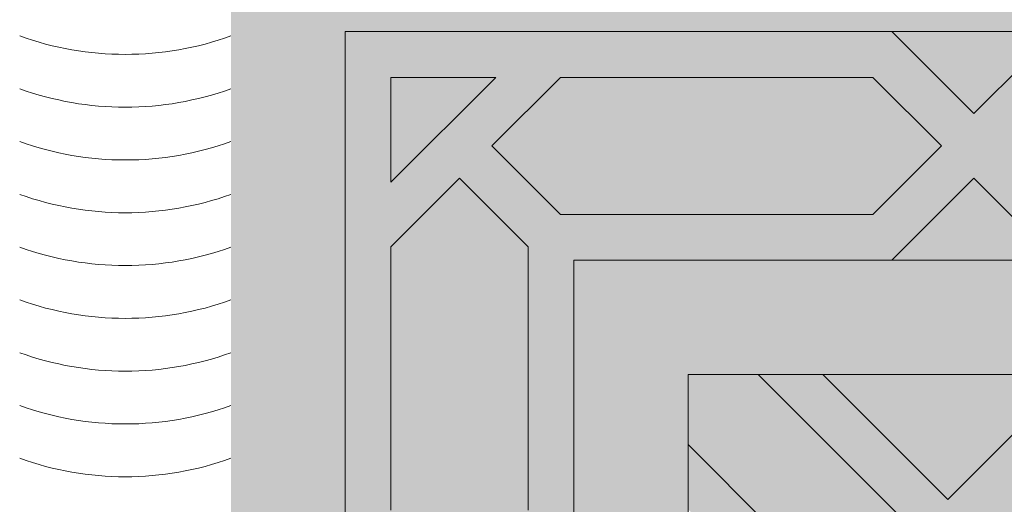
# Model space of a CAD drawing. Units: inches. Extents: x 844 to 2234, y 346 to 1084.
# Tile 58 of 93: x 1861.148 to 1866.641, y 710.205 to 712.909. Entities that reach past the tile are written whole.
import ezdxf

# ---------------------------------------------------------------- set-up
doc = ezdxf.new("R2010")
doc.units = ezdxf.units.IN
doc.header["$MEASUREMENT"] = 0
doc.layers.add('furniture', color=8, linetype='Continuous', lineweight=18)
doc.layers.add('RA-AP-01$0$INT', color=35, linetype='Continuous', lineweight=5)
doc.layers.add('RA-AP-01$0$FURN', color=3, linetype='Continuous')

# ---------------------------------------------------------------- blocks, each defined once
blk = doc.blocks.new('A$C18D01794')
at = {"layer": 'RA-AP-01$0$INT'}
h = blk.add_hatch(color=256, dxfattribs=at)
h.paths.add_polyline_path([(4.355206456958071, -6.156712009588037), (4.355206456958071, -8.056712009588038), (5.455206456958072, -8.056712009588038), (5.455206456958072, -6.156712009588037)])
h.paths.add_polyline_path([(4.405206456958072, -8.006712009588039), (4.405206456958072, -6.206712009588038), (5.405206456958072, -6.206712009588038), (5.405206456958072, -8.006712009588039)], flags=16)
h = blk.add_hatch(color=256, dxfattribs=at)
h.paths.add_polyline_path([(4.505206456958071, -7.585498806127123), (4.46934859260189, -7.549640941759413), (4.505206456958071, -7.513783077414768), (4.505206456958071, -7.381963272220687), (4.469348592616735, -7.346105407867824), (4.505206456958071, -7.310247543514964), (4.505206456958071, -7.178427738324996), (4.469348592586679, -7.142569873965138), (4.505206456952245, -7.106712009588038), (4.476922185709333, -7.106712009588038), (4.455206456960671, -7.128427738343681), (4.433490728198047, -7.106712009588038), (4.405206456946033, -7.106712009588036), (4.441064321339216, -7.142569873969684), (4.40520645695807, -7.178427738362358), (4.405206456958072, -7.310247543472698), (4.441064321364728, -7.346105407867826), (4.40520645695807, -7.381963272262947), (4.40520645695807, -7.513783077378263), (4.441064321354429, -7.549640941786153), (4.405206456958072, -7.585498806170974), (4.405206456958072, -7.717318611286652), (4.441064321333084, -7.753176475673194), (4.405206456958072, -7.789034340036673), (4.405206456958072, -8.006712009588039), (4.644348592588106, -8.006712009588039), (4.680206456964639, -7.970854145211967), (4.716064321341165, -8.006712009588039), (4.869348592586113, -8.006712009588039), (4.905206456964143, -7.970854145210465), (4.941064321342174, -8.006712009588039), (5.094348592587118, -8.006712009588037), (5.130206456963649, -7.970854145211967), (5.166064321340178, -8.006712009588039), (5.405206456958072, -8.006712009588039), (5.405206456958072, -7.789034340024526), (5.369348592595202, -7.753176475673196), (5.40520645695807, -7.717318611298797), (5.40520645695807, -7.585498806158829), (5.369348592573859, -7.549640941786151), (5.40520645695807, -7.51378307739041), (5.40520645695807, -7.381963272250803), (5.36934859256356, -7.346105407867824), (5.405206456958072, -7.310247543484846), (5.405206456958072, -7.178427738350217), (5.369348592589068, -7.142569873969682), (5.405206456982249, -7.106712009588038), (5.376922185730244, -7.106712009588038), (5.355206456967613, -7.128427738343679), (5.333490728218955, -7.10671200958804), (5.305206456976043, -7.106712009588042), (5.341064321341609, -7.142569873965136), (5.305206456958072, -7.178427738337141), (5.305206456958072, -7.310247543502816), (5.34106432131155, -7.346105407867824), (5.305206456958072, -7.381963272232832), (5.30520645695807, -7.513783077402624), (5.341064321326395, -7.549640941759413), (5.305206456958072, -7.585498806139263), (5.305206456958072, -7.717318611299605), (5.341064321347738, -7.753176475677737), (5.305206456958072, -7.78903434007894), (5.30520645695807, -7.906712009588039), (5.166064321336834, -7.906712009588039), (5.130206456963647, -7.942569873961684), (5.094348592590464, -7.906712009588039), (4.941064321338827, -7.906712009588041), (4.905206456964145, -7.942569873963183), (4.869348592589459, -7.906712009588039), (4.716064321337822, -7.906712009588041), (4.680206456964641, -7.942569873961684), (4.644348592591453, -7.906712009588039), (4.505206456958071, -7.906712009588039), (4.505206456958071, -7.789034340066795), (4.469348592580545, -7.753176475677738), (4.505206456958071, -7.717318611311748)])
h.paths.add_polyline_path([(4.485206456974132, -7.709034340046354), (4.45520645695909, -7.739034340051736), (4.425206456974128, -7.709034340057131), (4.425206456993394, -7.593783077384998), (4.45520645699153, -7.563783077396511), (4.485206456993396, -7.593783077408017)], flags=16)
h.paths.add_polyline_path([(4.455206456954537, -7.767318611299197), (4.485206456958242, -7.797318611312542), (4.48520645695951, -7.912569873958716), (4.45520645695415, -7.942569873954422), (4.425206456957888, -7.912569873967813), (4.425206456957888, -7.797318611286197)], flags=16)
h.paths.add_polyline_path([(4.455206456964794, -7.535498806149051), (4.42520645696469, -7.5054988061393), (4.425206456983954, -7.390247543486406), (4.455206456990734, -7.360247543489279), (4.485206456983953, -7.39024754349214), (4.485206456964687, -7.505498806158811)], flags=16)
h.paths.add_polyline_path([(4.499348592588947, -7.926712009585049), (4.636064321340932, -7.926712009585049), (4.666064321342317, -7.956712009586821), (4.636064321343707, -7.986712009585048), (4.499348592575121, -7.986712009585048), (4.469348592591685, -7.956712009591957)], flags=16)
h.paths.add_polyline_path([(4.425206456957888, -7.940854145195974), (4.471064321332215, -7.986712009585049), (4.425206456957888, -7.986712009585049)], flags=16)
h.paths.add_polyline_path([(4.455206456990734, -7.331963272246367), (4.425206456989053, -7.301963272254337), (4.425206456969784, -7.186712009596224), (4.455206456965226, -7.156712009591144), (4.485206456969787, -7.186712009586051), (4.485206456989053, -7.301963272238404)], flags=16)
h.paths.add_polyline_path([(4.72434859258714, -7.926712009586255), (4.861064321340141, -7.926712009586248), (4.891064321340324, -7.956712009586823), (4.861064321340513, -7.986712009586252), (4.724348592586768, -7.986712009586252), (4.694348592586956, -7.956712009586821)], flags=16)
h.paths.add_polyline_path([(4.919348592587961, -7.956712009586821), (4.949348592588145, -7.92671200958625), (5.08606432134115, -7.926712009586253), (5.116064321341327, -7.956712009586823), (5.086064321341519, -7.986712009586252), (4.949348592587774, -7.986712009586252)], flags=16)
h.paths.add_polyline_path([(5.144348592585967, -7.956712009586823), (5.174348592587358, -7.926712009585049), (5.311064321339338, -7.926712009585049), (5.3410643213366, -7.956712009591957), (5.311064321353163, -7.986712009585048), (5.174348592584576, -7.986712009585048)], flags=16)
h.paths.add_polyline_path([(5.32520645693489, -7.593783077408021), (5.355206456936755, -7.563783077396511), (5.385206456934894, -7.593783077384998), (5.38520645695416, -7.709034340057128), (5.355206456969194, -7.739034340051736), (5.325206456954153, -7.709034340046352)], flags=16)
h.paths.add_polyline_path([(5.325206456970042, -7.797318611312542), (5.355206456973747, -7.767318611299197), (5.385206456970398, -7.7973186112862), (5.385206456970398, -7.912569873967816), (5.355206456974136, -7.942569873954422), (5.325206456968778, -7.912569873958716)], flags=16)
h.paths.add_polyline_path([(5.325206456963599, -7.505498806158811), (5.325206456944333, -7.39024754349214), (5.355206456937552, -7.360247543489279), (5.385206456944332, -7.39024754348641), (5.385206456963596, -7.505498806139303), (5.355206456963492, -7.53549880614905)], flags=16)
h.paths.add_polyline_path([(5.32520645693923, -7.301963272238403), (5.3252064569585, -7.186712009586051), (5.355206456963062, -7.156712009591142), (5.3852064569585, -7.186712009596224), (5.385206456939234, -7.301963272254338), (5.355206456937552, -7.331963272246369)], flags=16)
h.paths.add_polyline_path([(5.339348592596071, -7.986712009585048), (5.385206456970398, -7.940854145195972), (5.385206456970396, -7.986712009585048)], flags=16)
h = blk.add_hatch(color=256, dxfattribs=at)
h.paths.add_polyline_path([(4.469348592586677, -7.142569873965136), (4.505206456958073, -7.178427738324996), (4.505206456958071, -7.106712009582215)])
h.paths.add_polyline_path([(4.455206456960671, -7.128427738343681), (4.476922185709333, -7.106712009588038), (4.433490728198045, -7.106712009588038)])
h.paths.add_polyline_path([(4.405206456958073, -7.178427738362358), (4.441064321339218, -7.142569873969684), (4.40520645695807, -7.106712009600073)])
h.paths.add_polyline_path([(4.425206456989053, -7.301963272254335), (4.455206456990736, -7.331963272246371), (4.485206456989055, -7.301963272238399), (4.48520645696979, -7.186712009586054), (4.455206456965227, -7.15671200959114), (4.425206456969784, -7.186712009596224)])
h.paths.add_polyline_path([(4.505206456958073, -7.381963272220689), (4.505206456958071, -7.310247543514961), (4.469348592616738, -7.346105407867826)])
h.paths.add_polyline_path([(4.425206456964688, -7.5054988061393), (4.455206456964794, -7.535498806149051), (4.485206456964689, -7.505498806158811), (4.485206456983951, -7.390247543492138), (4.455206456990736, -7.360247543489277), (4.425206456983956, -7.39024754348641)])
h.paths.add_polyline_path([(4.425206456974126, -7.709034340057128), (4.455206456959092, -7.739034340051736), (4.485206456974132, -7.709034340046356), (4.485206456993396, -7.593783077408017), (4.45520645699153, -7.563783077396511), (4.425206456993394, -7.593783077384999)])
h.paths.add_polyline_path([(4.46934859260189, -7.549640941759415), (4.505206456958071, -7.585498806127123), (4.505206456958073, -7.513783077414766)])
h.paths.add_polyline_path([(4.405206456958073, -7.585498806170972), (4.441064321354427, -7.549640941786151), (4.405206456958072, -7.513783077378263)])
h.paths.add_polyline_path([(4.405206456958072, -7.789034340036673), (4.441064321333084, -7.753176475673194), (4.405206456958072, -7.71731861128665)])
h.paths.add_polyline_path([(4.469348592580547, -7.75317647567774), (4.505206456958071, -7.789034340066795), (4.505206456958071, -7.717318611311744)])
h.paths.add_polyline_path([(4.425206456957888, -7.912569873967814), (4.45520645695415, -7.942569873954422), (4.485206456959507, -7.912569873958718), (4.48520645695824, -7.797318611312542), (4.455206456954537, -7.767318611299197), (4.425206456957888, -7.797318611286202)])
h.paths.add_polyline_path([(4.425206456957888, -7.986712009585049), (4.471064321332215, -7.986712009585049), (4.425206456957888, -7.940854145195972)])
h.paths.add_polyline_path([(4.499348592575121, -7.986712009585048), (4.636064321343707, -7.986712009585049), (4.666064321342317, -7.956712009586823), (4.636064321340932, -7.926712009585049), (4.499348592588945, -7.926712009585049), (4.469348592591685, -7.95671200959196)])
h.paths.add_polyline_path([(4.680206456964641, -7.942569873961684), (4.716064321337824, -7.906712009588039), (4.644348592591454, -7.906712009588039)])
h.paths.add_polyline_path([(4.644348592588108, -8.006712009588039), (4.716064321341167, -8.006712009588039), (4.680206456964637, -7.970854145211964)])
h.paths.add_polyline_path([(4.724348592586768, -7.98671200958625), (4.861064321340514, -7.986712009586252), (4.891064321340324, -7.956712009586819), (4.861064321340141, -7.92671200958625), (4.724348592587134, -7.926712009586255), (4.694348592586957, -7.956712009586821)])
h.paths.add_polyline_path([(4.905206456964143, -7.942569873963183), (4.941064321338827, -7.906712009588039), (4.869348592589457, -7.906712009588037)])
h.paths.add_polyline_path([(4.869348592586113, -8.006712009588039), (4.941064321342172, -8.006712009588037), (4.905206456964145, -7.970854145210463)])
h.paths.add_polyline_path([(4.949348592587774, -7.986712009586252), (5.086064321341521, -7.986712009586252), (5.116064321341329, -7.956712009586823), (5.08606432134115, -7.926712009586253), (4.949348592588145, -7.92671200958625), (4.919348592587961, -7.956712009586819)])
h.paths.add_polyline_path([(5.130206456963645, -7.942569873961684), (5.166064321336834, -7.906712009588039), (5.094348592590464, -7.906712009588039)])
h.paths.add_polyline_path([(5.094348592587119, -8.006712009588039), (5.166064321340178, -8.006712009588039), (5.130206456963651, -7.970854145211967)])
h.paths.add_polyline_path([(5.174348592584578, -7.986712009585048), (5.311064321353163, -7.986712009585048), (5.341064321336602, -7.956712009591958), (5.31106432133934, -7.926712009585049), (5.174348592587352, -7.926712009585049), (5.144348592585969, -7.956712009586823)])
h.paths.add_polyline_path([(5.325206456968778, -7.912569873958718), (5.355206456974136, -7.942569873954422), (5.385206456970396, -7.912569873967814), (5.385206456970396, -7.797318611286199), (5.355206456973747, -7.767318611299197), (5.325206456970044, -7.797318611312544)])
h.paths.add_polyline_path([(5.339348592596073, -7.986712009585048), (5.385206456970396, -7.986712009585049), (5.385206456970398, -7.94085414519597)])
h.paths.add_polyline_path([(5.325206456954155, -7.709034340046354), (5.355206456969194, -7.739034340051734), (5.38520645695416, -7.709034340057128), (5.385206456934896, -7.593783077384999), (5.355206456936758, -7.563783077396513), (5.325206456934888, -7.593783077408019)])
h.paths.add_polyline_path([(5.305206456958072, -7.789034340078938), (5.341064321347739, -7.753176475677738), (5.305206456958072, -7.717318611299605)])
h.paths.add_polyline_path([(5.369348592595204, -7.753176475673194), (5.40520645695807, -7.789034340024526), (5.405206456958072, -7.717318611298798)])
h.paths.add_polyline_path([(5.405206456958072, -7.585498806158831), (5.405206456958072, -7.513783077390407), (5.369348592573857, -7.549640941786151)])
h.paths.add_polyline_path([(5.305206456958072, -7.585498806139266), (5.341064321326393, -7.549640941759413), (5.305206456958072, -7.513783077402626)])
h.paths.add_polyline_path([(5.325206456963599, -7.50549880615881), (5.355206456963494, -7.535498806149055), (5.385206456963598, -7.505498806139302), (5.385206456944334, -7.390247543486411), (5.355206456937552, -7.360247543489279), (5.325206456944333, -7.39024754349214)])
h.paths.add_polyline_path([(5.305206456958072, -7.38196327223283), (5.341064321311551, -7.346105407867824), (5.305206456958072, -7.31024754350282)])
h.paths.add_polyline_path([(5.325206456939231, -7.301963272238404), (5.355206456937552, -7.331963272246369), (5.385206456939235, -7.301963272254335), (5.385206456958502, -7.186712009596224), (5.355206456963061, -7.156712009591142), (5.3252064569585, -7.186712009586051)])
h.paths.add_polyline_path([(5.404581768715993, -7.381338584008926, -0.001217816984214), (5.405206456958072, -7.381112009582329), (5.405206456958072, -7.310247543484846), (5.369348592563558, -7.346105407867826)])
h.paths.add_polyline_path([(5.36934859258907, -7.142569873969684), (5.40520645695807, -7.178427738350215), (5.405206456958072, -7.106712009612218)])
h.paths.add_polyline_path([(5.355206456967613, -7.128427738343683), (5.376922185730239, -7.106712009588038), (5.333490728218953, -7.10671200958804)])
h.paths.add_polyline_path([(5.30520645695807, -7.178427738337139), (5.341064321341609, -7.142569873965134), (5.305206456958074, -7.10671200957007)])
blk.add_hatch(color=256, dxfattribs=at).paths.add_polyline_path([(4.505206456958071, -7.906712009588039), (5.305206456958072, -7.906712009588039), (5.305206456958072, -7.106712009588038), (5.255206456951893, -7.106712009588036), (5.25520645694868, -7.856712009570104), (4.555206456959269, -7.856712009588616), (4.555206456956052, -7.106712009588038), (4.505206456958073, -7.106712009588038)])
h = blk.add_hatch(color=256, dxfattribs=at)
h.paths.add_polyline_path([(4.585917135068448, -7.856712009587804), (4.614201406330596, -7.856712009587056), (4.668846067270487, -7.802067348644738), (4.723490728212344, -7.856712009584164), (4.771774999457151, -7.856712009582887), (4.826419660396886, -7.80206734864072), (4.862780050090322, -7.838427738332541), (4.844495778842715, -7.856712009580965), (4.862780050090411, -7.856712009580482), (4.905206456960182, -7.814285602707865), (4.947632863832445, -7.856712009578238), (4.965917135079675, -7.856712009577755), (4.947632863831759, -7.838427738330656), (4.983993253523576, -7.802067348637219), (5.038637914464627, -7.856712009575829), (5.08692218571208, -7.856712009574554), (5.141566846649976, -7.802067348634224), (5.196211507589851, -7.856712009571666), (5.224495778822615, -7.856712009570916), (4.905206456953975, -7.537422687702283)])
h.paths.add_polyline_path([(4.895206456956031, -7.575706958950402), (4.895206456958921, -7.684996280828174), (4.840561796018589, -7.630351619890275)], flags=16)
h.paths.add_polyline_path([(4.915206456955638, -7.575706958949956), (4.969851117895509, -7.630351619887399), (4.915206456957609, -7.684996280827732)], flags=16)
h.paths.add_polyline_path([(4.826419660395175, -7.644493755514321), (4.881064321335613, -7.699138416452331), (4.771774999456703, -7.69913841645522)], flags=16)
h.paths.add_polyline_path([(4.983993253519558, -7.644493755510815), (5.038637914460456, -7.699138416449285), (4.929348592581548, -7.69913841645126)], flags=16)
h.paths.add_polyline_path([(4.881064321336025, -7.719138416452334), (4.826419660397532, -7.773783077393256), (4.771774999457062, -7.719138416455217)], flags=16)
h.paths.add_polyline_path([(4.929348592582019, -7.71913841645126), (5.038637914460982, -7.719138416449284), (4.983993253522945, -7.773783077389749)], flags=16)
h.paths.add_polyline_path([(4.895206456960191, -7.733280552075633), (4.895206456962115, -7.806001331460164), (4.876922185715016, -7.824285602708492), (4.840561796021581, -7.787925213016675)], flags=16)
h.paths.add_polyline_path([(4.915206456958487, -7.733280552075187), (4.969851117899527, -7.787925213013798), (4.933490728206909, -7.824285602708034), (4.9152064569598, -7.806001331461736)], flags=16)
h.paths.add_polyline_path([(4.757632863832376, -7.733280552079264), (4.812277524772842, -7.787925213017304), (4.757632863834348, -7.842569873958233)], flags=16)
h.paths.add_polyline_path([(4.737632863832376, -7.73328055207979), (4.737632863834348, -7.842569873958701), (4.682988202893906, -7.787925213020692)], flags=16)
h.paths.add_polyline_path([(5.05278005008503, -7.733280552072701), (5.052780050087917, -7.842569873951664), (4.998135389146995, -7.787925213013169)], flags=16)
h.paths.add_polyline_path([(5.072780050085024, -7.733280552072333), (5.127424711025931, -7.787925213010806), (5.072780050087916, -7.842569873951244)], flags=16)
h.paths.add_polyline_path([(4.935917135072783, -7.506712009583784), (5.255206456948811, -7.826001331459767), (5.255206456948932, -7.797717060211899), (5.200561796010279, -7.743072399273238), (5.255206456949403, -7.688427738334128), (5.25520645694961, -7.640143467086677), (5.200561796009787, -7.585498806146837), (5.236922185702417, -7.549138416454212), (5.255206456949919, -7.56742268770172), (5.255206456949998, -7.549138416454178), (5.212780050078687, -7.506712009583814), (5.25520645695036, -7.464285602712145), (5.255206456950438, -7.446001331464763), (5.236922185702424, -7.464285602712779), (5.200561796009796, -7.427925213020149), (5.255206456950753, -7.373280552079203), (5.25520645695096, -7.324996280834394), (5.200561796010322, -7.270351619893748), (5.255206456951428, -7.215706958952649), (5.255206456951547, -7.187422687705071)])
h.paths.add_polyline_path([(5.042988202883395, -7.42792521302065), (5.097632863823085, -7.373280552080975), (5.097632863822622, -7.482569873959883)], flags=16)
h.paths.add_polyline_path([(5.028846067259663, -7.442067348644384), (5.083490728198774, -7.496712009583504), (4.974201406321001, -7.496712009583035)], flags=16)
h.paths.add_polyline_path([(5.117632863823087, -7.37328055208089), (5.172277524762331, -7.42792521302015), (5.11763286382262, -7.482569873959851)], flags=16)
h.paths.add_polyline_path([(5.08349072819877, -7.516712009582191), (5.028846067259652, -7.571356670521302), (4.974201406320998, -7.516712009582638)], flags=16)
h.paths.add_polyline_path([(5.131774999446817, -7.35913841645716), (5.186419660386065, -7.413783077396415), (5.241064321325782, -7.359138416456712)], flags=17)
h.paths.add_polyline_path([(5.131774999446228, -7.496712009583703), (5.186419660386065, -7.442067348643883), (5.222780050079488, -7.478427738337313), (5.204495778832781, -7.496712009584014)], flags=16)
h.paths.add_polyline_path([(5.097632863822613, -7.530854145205813), (5.097632863823061, -7.640143467084723), (5.042988202883383, -7.585498806145032)], flags=16)
h.paths.add_polyline_path([(5.131774999446899, -7.339138416457162), (5.241064321325809, -7.339138416456712), (5.186419660386591, -7.284493755517479)], flags=17)
h.paths.add_polyline_path([(5.131774999446226, -7.516712009581999), (5.204495778830767, -7.516712009581702), (5.22278005007868, -7.534996280829206), (5.186419660386049, -7.571356670521828)], flags=16)
h.paths.add_polyline_path([(5.11763286382262, -7.530854145205852), (5.17227752476232, -7.585498806145562), (5.117632863823064, -7.64014346708481)], flags=16)
h.paths.add_polyline_path([(5.186419660386069, -7.599640941770585), (5.241064321325754, -7.654285602710281), (5.131774999446791, -7.654285602709814)], flags=16)
h.paths.add_polyline_path([(5.131774999446872, -7.674285602709813), (5.24106432132578, -7.674285602710282), (5.186419660386554, -7.728930263649504)], flags=16)
h.paths.add_polyline_path([(5.255206456951811, -7.126001331467467), (5.255206456951895, -7.106712009588038), (4.555206456956052, -7.106712009588038), (4.555206456956136, -7.12600133146746), (4.905206456953973, -7.476001331465289)])
h.paths.add_polyline_path([(4.983993253513404, -7.368930263651977), (4.92934859257295, -7.314285602713969), (5.03863791445186, -7.314285602711063)], flags=16)
h.paths.add_polyline_path([(4.969851117889988, -7.383072399276016), (4.915206456952556, -7.437717060215906), (4.915206456949648, -7.328427738338133)], flags=16)
h.paths.add_polyline_path([(4.929348592572535, -7.294285602713971), (4.983993253511019, -7.239640941773039), (5.038637914451496, -7.294285602711065)], flags=16)
h.paths.add_polyline_path([(5.052780050074912, -7.280143467087016), (4.998135389134438, -7.225498806148989), (5.052780050072919, -7.170854145208052)], flags=16)
h.paths.add_polyline_path([(5.07278005007491, -7.280143467086489), (5.072780050072918, -7.170854145207579), (5.127424711013374, -7.225498806145578)], flags=16)
h.paths.add_polyline_path([(4.89520645695295, -7.437717060216355), (4.840561796013067, -7.383072399278919), (4.895206456950961, -7.328427738338582)], flags=16)
h.paths.add_polyline_path([(4.915206456948365, -7.280143467090674), (4.915206456946434, -7.207422687704125), (4.933490728192729, -7.18913841645701), (4.969851117886972, -7.225498806149623)], flags=16)
h.paths.add_polyline_path([(4.881064321327021, -7.314285602715054), (4.82641966038902, -7.368930263655506), (4.771774999448108, -7.314285602717047)], flags=16)
h.paths.add_polyline_path([(4.895206456950073, -7.280143467091125), (4.840561796009022, -7.225498806152518), (4.876922185700835, -7.18913841645908), (4.895206456948749, -7.207422687706589)], flags=16)
h.paths.add_polyline_path([(4.983993253510392, -7.211356670525576), (4.947632863816944, -7.174996280833758), (4.965917135064043, -7.156712009585847), (5.038637914448995, -7.156712009584522)], flags=16)
h.paths.add_polyline_path([(4.881064321326543, -7.294285602715056), (4.771774999447578, -7.294285602717046), (4.826419660385607, -7.239640941776569)], flags=16)
h.paths.add_polyline_path([(4.905206456946447, -7.19913841645844), (4.862780050074785, -7.156712009587725), (4.947632863816685, -7.156712009586302)], flags=16)
h.paths.add_polyline_path([(5.14156684663679, -7.211356670521528), (5.086922185696452, -7.156712009583639), (5.196211507574223, -7.156712009581651)], flags=16)
h.paths.add_polyline_path([(4.8264196603837, -7.211356670529104), (4.771774999442643, -7.156712009590501), (4.8444957788276, -7.156712009588568), (4.862780050075511, -7.17499628083566)], flags=16)
h.paths.add_polyline_path([(4.812277524760289, -7.225498806153156), (4.757632863822258, -7.28014346709363), (4.757632863819352, -7.170854145214669)], flags=16)
h.paths.add_polyline_path([(4.73763286382226, -7.280143467093997), (4.682988202881349, -7.22549880615554), (4.737632863819352, -7.170854145215086)], flags=16)
h.paths.add_polyline_path([(4.723490728195188, -7.156712009591787), (4.668846067257299, -7.211356670532127), (4.614201406317417, -7.156712009594693)], flags=16)
h.paths.add_polyline_path([(4.597632863829262, -7.506712009583814), (4.555206456957951, -7.54913841645418), (4.555206456958029, -7.56742268770172), (4.573490728205535, -7.549138416454212), (4.609851117898167, -7.585498806146839), (4.555206456958338, -7.640143467086675), (4.555206456958546, -7.688427738334125), (4.60985111789767, -7.743072399273238), (4.555206456959015, -7.797717060211899), (4.555206456959138, -7.826001331459767), (4.874495778835167, -7.506712009583786), (4.5552064569564, -7.187422687705062), (4.555206456956523, -7.215706958952644), (4.609851117897629, -7.270351619893746), (4.555206456956988, -7.324996280834396), (4.555206456957198, -7.373280552079195), (4.609851117898153, -7.427925213020147), (4.573490728205528, -7.464285602712779), (4.555206456957507, -7.446001331464756), (4.555206456957585, -7.464285602712143)])
h.paths.add_polyline_path([(4.712780050085332, -7.482569873959882), (4.712780050084863, -7.373280552080972), (4.767424711024555, -7.42792521302065)], flags=16)
h.paths.add_polyline_path([(4.726922185709173, -7.496712009583504), (4.781566846648288, -7.442067348644384), (4.836211507586949, -7.496712009583033)], flags=16)
h.paths.add_polyline_path([(4.692780050085327, -7.482569873959851), (4.638135389145619, -7.427925213020149), (4.692780050084865, -7.373280552080892)], flags=16)
h.paths.add_polyline_path([(4.726922185709182, -7.516712009582191), (4.836211507586949, -7.51671200958264), (4.7815668466483, -7.571356670521304)], flags=16)
h.paths.add_polyline_path([(4.678637914461726, -7.496712009583706), (4.605917135075169, -7.496712009584014), (4.587632863828464, -7.478427738337311), (4.623993253521887, -7.442067348643881)], flags=16)
h.paths.add_polyline_path([(4.712780050085336, -7.530854145205816), (4.767424711024568, -7.585498806145034), (4.71278005008489, -7.640143467084724)], flags=16)
h.paths.add_polyline_path([(4.678637914461726, -7.516712009582001), (4.623993253521899, -7.571356670521829), (4.587632863829271, -7.534996280829206), (4.605917135077185, -7.5167120095817)], flags=16)
h.paths.add_polyline_path([(4.692780050085336, -7.530854145205848), (4.692780050084889, -7.64014346708481), (4.638135389145632, -7.585498806145562)], flags=16)
h.paths.add_polyline_path([(4.623993253521885, -7.413783077396415), (4.678637914461131, -7.359138416457161), (4.56934859258217, -7.359138416456712)], flags=17)
h.paths.add_polyline_path([(4.623993253521901, -7.599640941770568), (4.678637914461158, -7.654285602709814), (4.569348592582195, -7.654285602710281)], flags=16)
h.paths.add_polyline_path([(4.678637914461051, -7.339138416457162), (4.623993253521361, -7.284493755517479), (4.569348592582143, -7.339138416456712)], flags=17)
h.paths.add_polyline_path([(4.678637914461076, -7.674285602709813), (4.623993253521399, -7.728930263649504), (4.569348592582167, -7.674285602710281)], flags=16)
h = blk.add_hatch(color=256, dxfattribs=at)
h.paths.add_polyline_path([(4.905206456954232, -7.537422687702028), (4.874495778835232, -7.506712009583718), (4.555206456959138, -7.826001331459766), (4.555206456959269, -7.856712009588616), (4.585917135068449, -7.856712009587804)])
h.paths.add_polyline_path([(4.935917135072152, -7.506712009583152), (4.905206456953497, -7.537422687701806), (5.224495778822614, -7.856712009570917), (5.255206456948681, -7.856712009570104), (5.255206456948813, -7.826001331459768)])
h.paths.add_polyline_path([(5.255206456951549, -7.18742268770507), (5.255206456951813, -7.126001331467461), (4.905206456953563, -7.476001331465701), (4.935917135072559, -7.506712009584006)])
h.paths.add_polyline_path([(4.874495778835167, -7.506712009583785), (4.905206456953818, -7.476001331465132), (4.555206456956135, -7.126001331467458), (4.555206456956399, -7.187422687705064)])
h = blk.add_hatch(color=256, dxfattribs=at)
h.paths.add_polyline_path([(4.969851117891331, -7.630351619889621), (4.915206456952669, -7.575706958950966), (4.915206456952222, -7.684996280828739)])
h.paths.add_polyline_path([(4.895206456953064, -7.575706958950968), (4.840561796014413, -7.630351619889628), (4.895206456953533, -7.684996280828741)])
h.paths.add_polyline_path([(4.826419660390684, -7.644493755513362), (4.771774999451003, -7.699138416453052), (4.881064321329913, -7.699138416452587)])
h.paths.add_polyline_path([(4.881064321329884, -7.719138416452585), (4.771774999450921, -7.719138416453052), (4.82641966039018, -7.773783077392298)])
h.paths.add_polyline_path([(4.895206456953734, -7.733280552076196), (4.840561796013912, -7.787925213016031), (4.876922185707337, -7.824285602709455), (4.895206456954043, -7.806001331462747)])
h.paths.add_polyline_path([(4.862780050082808, -7.838427738332388), (4.826419660390178, -7.802067348639763), (4.771774999450351, -7.856712009579595), (4.844495778835303, -7.856712009579895)])
h.paths.add_polyline_path([(4.812277524766446, -7.787925213016036), (4.757632863827191, -7.733280552076788), (4.757632863826741, -7.842569873955747)])
h.paths.add_polyline_path([(4.737632863827191, -7.733280552076863), (4.682988202887508, -7.787925213016558), (4.737632863826743, -7.842569873955778)])
h.paths.add_polyline_path([(4.668846067263777, -7.802067348640287), (4.614201406325123, -7.856712009578949), (4.723490728202894, -7.856712009579402)])
h.paths.add_polyline_path([(4.905206456953846, -7.814285602708654), (4.862780050082654, -7.856712009579847), (4.947632863824561, -7.85671200958032)])
h.paths.add_polyline_path([(4.915206456952028, -7.733280552076195), (4.91520645695173, -7.806001331460731), (4.933490728199234, -7.824285602708648), (4.96985111789186, -7.787925213016022)])
h.paths.add_polyline_path([(5.038637914454841, -7.719138416453029), (4.929348592575874, -7.71913841645258), (4.983993253515593, -7.773783077392289)])
h.paths.add_polyline_path([(4.983993253515065, -7.644493755513352), (4.929348592575849, -7.699138416452582), (5.038637914454755, -7.699138416453031)])
h.paths.add_polyline_path([(5.052780050079843, -7.73328055207676), (4.998135389140595, -7.787925213016018), (5.052780050080309, -7.842569873955721)])
h.paths.add_polyline_path([(4.983993253516868, -7.802067348639752), (4.947632863824241, -7.838427738332383), (4.965917135071747, -7.856712009579888), (5.038637914456701, -7.856712009579572)])
h.paths.add_polyline_path([(5.127424711019533, -7.787925213016519), (5.072780050079843, -7.733280552076838), (5.07278005008031, -7.842569873955751)])
h.paths.add_polyline_path([(5.141566846643269, -7.802067348640248), (5.086922185704154, -7.85671200957937), (5.196211507581929, -7.856712009578901)])
for p, q in [((4.555206456956052, -7.106712009588036), (4.555206456959269, -7.856712009588616)), ((4.874495778835167, -7.506712009583786), (4.555206456959136, -7.826001331459769)), ((4.905206456953975, -7.537422687702283), (4.585917135071132, -7.856712009585121)), ((4.425206456957888, -7.797318611286199), (4.425206456957888, -7.912569873967814)), ((4.485206456959509, -7.912569873958718), (4.485206456958242, -7.797318611312544)), ((4.614201406333045, -7.85671200958461), (4.668846067270487, -7.802067348644737)), ((4.723490728210815, -7.856712009582635), (4.668846067270487, -7.802067348644737)), ((4.555206456959269, -7.856712009588616), (5.255206456948681, -7.856712009570104)), ((5.267206456961765, -7.906712009586254), (4.543206456966523, -7.906712009586254)), ((5.2672064569642, -7.906712009586255), (4.54320645696085, -7.906712009586255)), ((4.644348592589667, -7.906712009586254), (4.680206456964639, -7.942569873961684)), ((4.716064321339607, -7.906712009586254), (4.680206456964639, -7.942569873961684)), ((4.425206456957888, -7.912569873967814), (4.45520645695415, -7.942569873954422)), ((4.485206456959509, -7.912569873958718), (4.45520645695415, -7.942569873954422)), ((4.499348592588947, -7.926712009585049), (4.469348592591685, -7.956712009591957)), ((4.636064321340932, -7.926712009585049), (4.499348592588947, -7.926712009585049)), ((4.636064321340932, -7.926712009585049), (4.666064321342317, -7.956712009586823)), ((4.425206456957888, -7.940854145195974), (4.425206456957888, -7.986712009585049)), ((4.471064321332213, -7.986712009585048), (4.425206456957888, -7.940854145195974)), ((4.499348592575123, -7.986712009585048), (4.469348592591685, -7.956712009591957)), ((4.636064321343709, -7.986712009585049), (4.666064321342317, -7.956712009586823)), ((4.644348592589893, -8.006712009586252), (4.680206456964637, -7.970854145211966)), ((4.716064321339382, -8.006712009586252), (4.680206456964637, -7.970854145211966)), ((4.471064321332213, -7.986712009585048), (4.425206456957888, -7.986712009585049)), ((4.636064321343709, -7.986712009585049), (4.499348592575123, -7.986712009585048))]:
    blk.add_line(p, q, dxfattribs=at)
for points in [[(5.405206456958072, -8.006712009588039), (4.405206456958072, -8.006712009588039), (4.405206456958072, -7.106712009588038)], [(5.305206456958072, -7.106712009588038), (5.305206456958072, -7.906712009588039), (4.505206456958071, -7.906712009588039), (4.505206456958071, -7.106712009588038)]]:
    blk.add_lwpolyline(points, dxfattribs=at)
for centre in [(4.309006456952313, -7.948364458284338), (4.309006456952086, -7.971464458286042), (4.30900645694913, -7.994564458281608), (4.309006456948902, -8.017664458286497), (4.309006456951858, -8.040764458285018), (4.309006456950267, -8.063864458283767), (4.309006456948448, -8.086964458285472), (4.309006456948448, -8.11006445828422), (4.309006456946856, -8.13316445828297)]:
    blk.add_arc(centre, 0.136414042854523, 70.20384312815696, 109.7961568705686, dxfattribs=at)
blk = doc.blocks.new('A$C5D2F253E')
at = {"layer": 'RA-AP-01$0$FURN', "xscale": -0.7999999999883585, "yscale": 0.7999999999883585, "zscale": 0.8, "rotation": 90}
blk.add_blockref('A$C18D01794', (-5.687757199772477, 4.75791982714071), dxfattribs=at)

msp = doc.modelspace()

# ---------------------------------------------------------------- block references
at = {"layer": 'furniture', "xscale": 15.94108302203742, "yscale": 15.94108302203742, "zscale": 15.94108302203742, "rotation": 90}
msp.add_blockref('A$C5D2F253E', (1882.631064852549, 701.4028671565849), dxfattribs=at)

doc.saveas('drawing.dxf')
